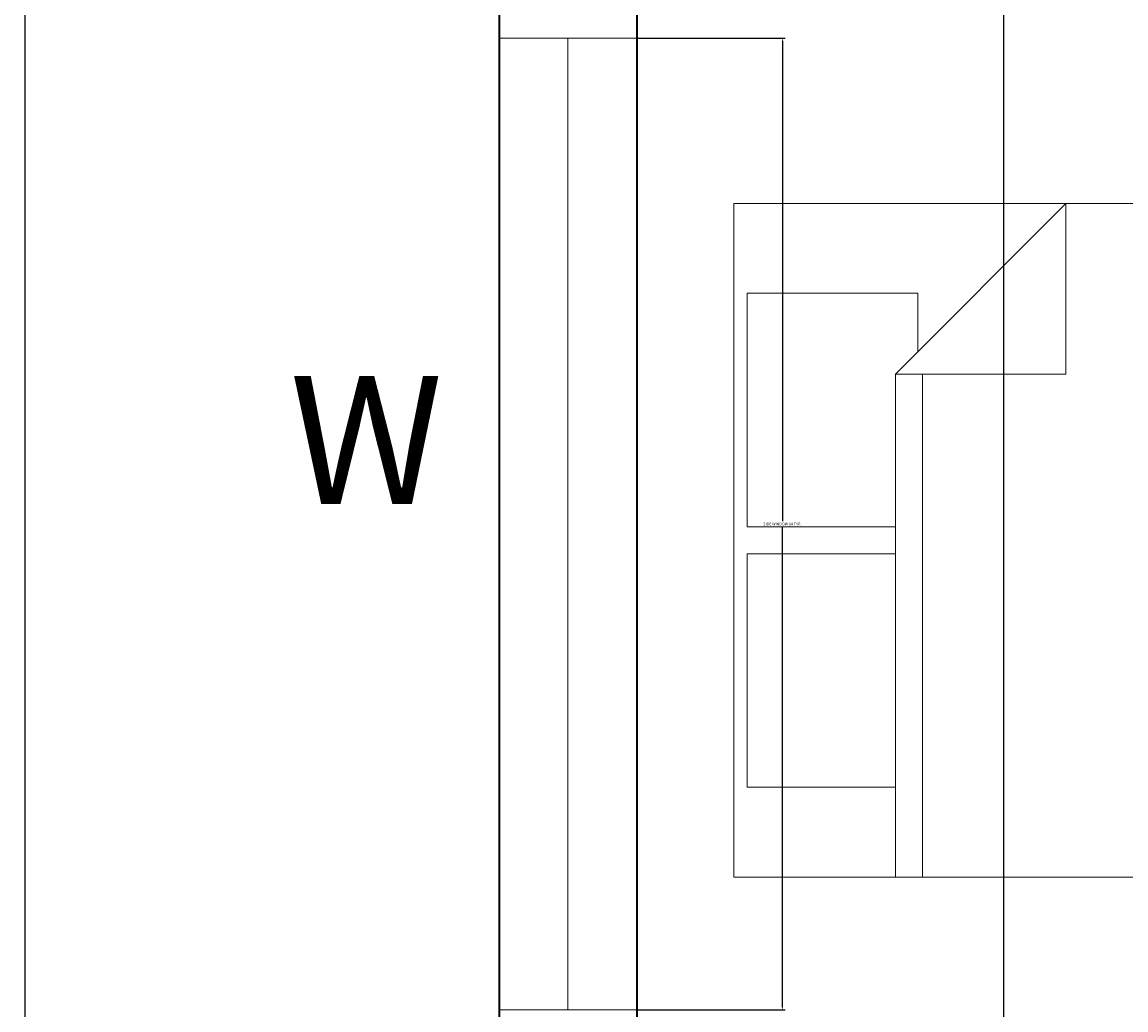
# Model space of a CAD drawing. Units: feet. Extents: x 1654 to 2985, y 1348 to 2230.
# Tile 2 of 53: x 1812 to 1884, y 1641 to 1706. Entities that reach past the tile are written whole.
import ezdxf

# ---------------------------------------------------------------- set-up
doc = ezdxf.new("R2010")
doc.units = ezdxf.units.FT
for name, color, linetype, lineweight in [('A-ANNO-DIMS', 2, 'Continuous', 18), ('A-ANNO-TEXT', 7, 'Continuous', 18), ('A-FURN', 8, 'Continuous', 13), ('A-GLAZ', 4, 'Continuous', 18), ('A-WALL', 7, 'Continuous', 35)]:
    doc.layers.add(name, color=color, linetype=linetype, lineweight=lineweight)
doc.styles.get("Standard").update_dxf_attribs({"font": 'arial.ttf'})
doc.dimstyles.get("Standard").update_dxf_attribs({"dimtxt": 0.18, "dimasz": 0.18, "dimexe": 0.18, "dimexo": 0.0625, "dimgap": 0.09, "dimtad": 0, "dimtih": 1, "dimtoh": 1, "dimdec": 4, "dimzin": 0, "dimdsep": 46, "dimtxsty": 'Standard', "dimcen": 0.09, "dimadec": 0, "dimazin": 0, "dimtfac": 1, "dimtdec": 4, "dimtofl": 0, "dimtmove": 0, "dimatfit": 3, "dimfxl": 1, "dimtolj": 1, "dimtzin": 0, "dimarcsym": 0})

# ---------------------------------------------------------------- blocks, each defined once
blk = doc.blocks.new('Bed - Queen')
for p, q in [((0, -80.00003), (0, 0)), ((0, 0), (59.99999, 0)), ((59.99999, 0), (59.99999, -80.00003)), ((7.99999, -1.2), (28.79998, -1.2)), ((7.99999, -14.4), (7.99999, -1.2)), ((28.79998, -1.2), (28.79998, -14.4)), ((31.19999, -1.2), (51.99999, -1.2)), ((31.19999, -14.4), (31.19999, -1.2)), ((51.99999, -1.2), (51.99999, -16.4)), ((0, -14.4), (44.8, -14.4)), ((59.99999, -29.6), (44.8, -14.4)), ((44.8, -14.4), (44.8, -29.6)), ((51.99999, -16.4), (46.79936, -16.4)), ((44.8, -16.8), (0, -16.8)), ((44.8, -29.6), (59.99999, -29.6)), ((59.99999, -80.00003), (0, -80.00003))]:
    blk.add_line(p, q)
blk = doc.blocks.new('WIN-GUEST-SIDE')
for p, q in [((0, 63.534), (9, 63.534)), ((4.5, 63.534), (4.5, 0)), ((9, 0), (0, 0))]:
    blk.add_line(p, q)
blk = doc.blocks.new('*D64')
at = {"layer": 'A-ANNO-DIMS', "color": 0, "lineweight": -2, "transparency": 16777216}
for p, q in [((1852.155, 1704.721), (1861.803, 1704.721)), ((1861.623, 1704.541), (1861.623, 1673.137)), ((1861.623, 1641.367), (1861.623, 1672.771)), ((1852.155, 1641.187), (1861.803, 1641.187))]:
    blk.add_line(p, q, dxfattribs=at)
at = {"layer": 'A-ANNO-DIMS', "color": 0, "transparency": 16777216}
for points in [[(1861.593, 1704.541), (1861.653, 1704.541), (1861.623, 1704.721)], [(1861.593, 1641.367), (1861.653, 1641.367), (1861.623, 1641.187)]]:
    blk.add_solid(points, dxfattribs=at)
at = {"layer": 'Defpoints', "color": 0, "transparency": 16777216}
for p in [(1852.092, 1704.721), (1861.623, 1704.721), (1852.092, 1641.187)]:
    blk.add_point(p, dxfattribs=at)
at = {"layer": 'A-ANNO-DIMS', "color": 0, "transparency": 16777216, "insert": (1861.623, 1672.954), "char_height": 0.18, "attachment_point": 5}
blk.add_mtext('\\A1;SIDE WINDOW 64 TYP.', dxfattribs=at)
blk = doc.blocks.new('*D65')
at = {"layer": 'A-ANNO-DIMS', "color": 0, "lineweight": -2, "transparency": 16777216}
for p, q in [((1843.092, 1641.124), (1843.092, 1631.477)), ((1852.092, 1641.124), (1852.092, 1631.477)), ((1843.272, 1631.657), (1847.134, 1631.657)), ((1851.912, 1631.657), (1848.051, 1631.657))]:
    blk.add_line(p, q, dxfattribs=at)
at = {"layer": 'A-ANNO-DIMS', "color": 0, "transparency": 16777216}
for points in [[(1843.272, 1631.687), (1843.272, 1631.627), (1843.092, 1631.657)], [(1851.912, 1631.687), (1851.912, 1631.627), (1852.092, 1631.657)]]:
    blk.add_solid(points, dxfattribs=at)
at = {"layer": 'Defpoints', "color": 0, "transparency": 16777216}
for p in [(1843.092, 1641.187), (1852.092, 1641.187), (1852.092, 1631.657)]:
    blk.add_point(p, dxfattribs=at)
at = {"layer": 'A-ANNO-DIMS', "color": 0, "transparency": 16777216, "insert": (1847.592, 1631.657), "char_height": 0.18, "attachment_point": 5}
blk.add_mtext('\\A1;9 TYP.', dxfattribs=at)
blk = doc.blocks.new('*D77')
at = {"layer": 'A-ANNO-DIMS', "color": 0, "lineweight": -2, "transparency": 16777216}
for p, q in [((1843.03, 2117.255), (1811.912, 2117.255)), ((1812.092, 2117.075), (1812.092, 1841.437)), ((1812.092, 1565.435), (1812.092, 1841.073)), ((1843.03, 1565.255), (1811.912, 1565.255))]:
    blk.add_line(p, q, dxfattribs=at)
at = {"layer": 'A-ANNO-DIMS', "color": 0, "transparency": 16777216}
for points in [[(1812.062, 2117.075), (1812.122, 2117.075), (1812.092, 2117.255)], [(1812.062, 1565.435), (1812.122, 1565.435), (1812.092, 1565.255)]]:
    blk.add_solid(points, dxfattribs=at)
at = {"layer": 'Defpoints', "color": 0, "transparency": 16777216}
for p in [(1812.092, 2117.255), (1843.092, 2117.255), (1843.092, 1565.255)]:
    blk.add_point(p, dxfattribs=at)
at = {"layer": 'A-ANNO-DIMS', "color": 0, "transparency": 16777216, "insert": (1812.092, 1841.255), "char_height": 0.18, "attachment_point": 5}
blk.add_mtext('\\A1;552', dxfattribs=at)
blk = doc.blocks.new('*D100')
at = {"layer": 'A-ANNO-DIMS', "color": 0, "lineweight": -2, "transparency": 16777216}
for p, q in [((1852.092, 1751.192), (1852.092, 1534.075)), ((1876.092, 1751.192), (1876.092, 1534.075)), ((1852.272, 1534.255), (1863.872, 1534.255)), ((1875.912, 1534.255), (1864.313, 1534.255))]:
    blk.add_line(p, q, dxfattribs=at)
at = {"layer": 'A-ANNO-DIMS', "color": 0, "transparency": 16777216}
for points in [[(1852.272, 1534.285), (1852.272, 1534.225), (1852.092, 1534.255)], [(1875.912, 1534.285), (1875.912, 1534.225), (1876.092, 1534.255)]]:
    blk.add_solid(points, dxfattribs=at)
at = {"layer": 'Defpoints', "color": 0, "transparency": 16777216}
for p in [(1852.092, 1751.255), (1876.092, 1751.255), (1876.092, 1534.255)]:
    blk.add_point(p, dxfattribs=at)
at = {"layer": 'A-ANNO-DIMS', "color": 0, "transparency": 16777216, "insert": (1864.092, 1534.255), "char_height": 0.18, "attachment_point": 5}
blk.add_mtext('\\A1;24', dxfattribs=at)

msp = doc.modelspace()

# ---------------------------------------------------------------- linework, layer by layer
at = {"layer": 'A-WALL'}
for p, q in [((1843.0924, 2117.2549), (1843.0924, 1565.2549)), ((1843.0924, 1742.2549), (1843.0924, 1565.2549)), ((1852.0924, 1742.2549), (1852.0924, 1574.2549))]:
    msp.add_line(p, q, dxfattribs=at)

# ---------------------------------------------------------------- block references
at = {"layer": 'A-FURN', "xscale": 0.7339343441631778, "yscale": 0.7339343441631778, "zscale": 0.7339343441631778, "rotation": 90}
msp.add_blockref('Bed - Queen', (1858.4494, 1649.8757), dxfattribs=at)
at = {"layer": 'A-GLAZ'}
msp.add_blockref('WIN-GUEST-SIDE', (1843.092, 1641.187), dxfattribs=at)

# ---------------------------------------------------------------- texts
at = {"layer": 'A-ANNO-TEXT'}
msp.add_text('W', height=8.3811, dxfattribs=at).set_placement((1829.3876, 1674.2554))

# ---------------------------------------------------------------- dimensions: what is measured, and where the dimension line sits
at = {"layer": 'A-ANNO-DIMS'}
dim = msp.add_linear_dim(base=(1812.0924, 2117.2549), p1=(1843.0924, 1565.2549), p2=(1843.0924, 2117.2549), angle=90, dimstyle='Standard', override={"dimdec": 0, "dimlfac": 1, "dimrnd": 0, "dimzin": 0, "dimdsep": 46, "dimlunit": 2}, dxfattribs=at)
dim.commit()
dim.dimension.update_dxf_attribs({"geometry": '*D77', "text_midpoint": (1812.0924, 1841.2549)})
dim = msp.add_linear_dim(base=(1876.0924, 1534.2549), p1=(1852.0924, 1751.2549), p2=(1876.0924, 1751.2549), dimstyle='Standard', override={"dimdec": 0, "dimlfac": 1, "dimrnd": 0, "dimzin": 0, "dimdsep": 46, "dimlunit": 2}, dxfattribs=at)
dim.commit()
dim.dimension.update_dxf_attribs({"geometry": '*D100', "text_midpoint": (1864.0924, 1534.2549)})
dim = msp.add_linear_dim(base=(1861.6225, 1704.7209), p1=(1852.0924, 1641.187), p2=(1852.0924, 1704.7209), angle=90, text='SIDE WINDOW <> TYP.', dimstyle='Standard', override={"dimdec": 0, "dimlfac": 1, "dimrnd": 0, "dimzin": 0, "dimdsep": 46, "dimlunit": 2}, dxfattribs=at)
dim.commit()
dim.dimension.update_dxf_attribs({"geometry": '*D64', "text_midpoint": (1861.6225, 1672.954)})
dim = msp.add_linear_dim(base=(1852.0924, 1631.6569), p1=(1843.0924, 1641.187), p2=(1852.0924, 1641.187), text='<> TYP.', dimstyle='Standard', override={"dimdec": 0, "dimlfac": 1, "dimrnd": 0, "dimzin": 0, "dimdsep": 46, "dimlunit": 2}, dxfattribs=at)
dim.commit()
dim.dimension.update_dxf_attribs({"geometry": '*D65', "text_midpoint": (1847.5924, 1631.6569)})

doc.saveas('drawing.dxf')
